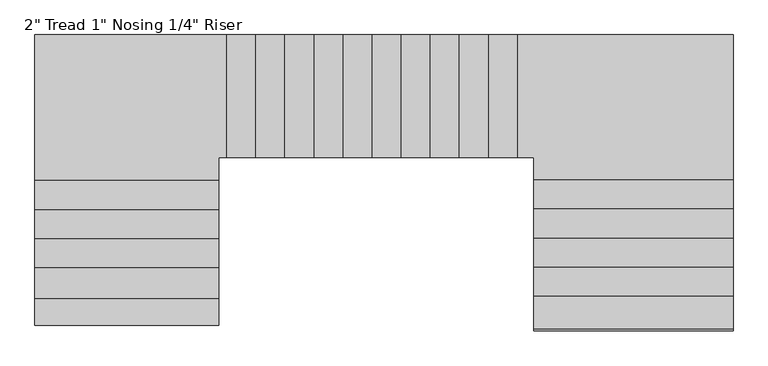
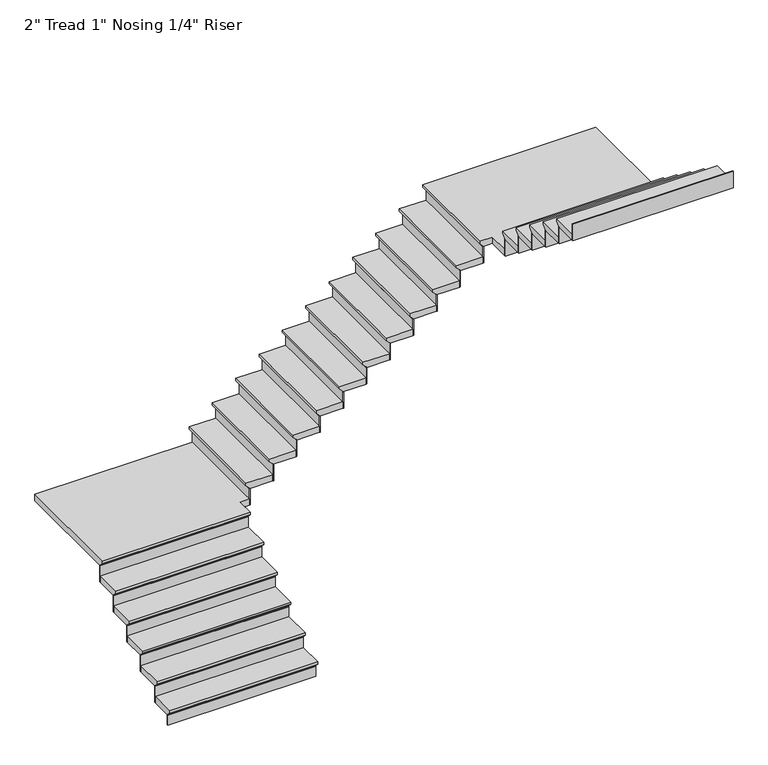
"""IFC4 building model written with IfcOpenShell, lengths in millimetres: stair flight geometry."""

from ifc_helpers import new_model, si_unit, origin, place, context, project, spatial, faceted_brep, source, transform, mapped, element, save


def stair_flight_6a7f422e(model_context):
    return source(origin(), model_context, "Body", "Brep", [
        faceted_brep([(-2368.6972892, 4718.9167606, 12915.0717391), (-2368.6972892, 4718.9167606, 12934.1217391), (-3493.0046642, 4718.9167606, 12934.1217391), (-3493.0046642, 4718.9167606, 12915.0717391), (-2368.6972892, 4744.3167606, 12889.6717391), (-3493.0046642, 4744.3167606, 12889.6717391), (-2368.6972892, 4909.4167606, 12934.1217391), (-3493.0046642, 4909.4167606, 12934.1217391), (-3493.0046642, 4744.3167606, 12883.3217391), (-3493.0046642, 4909.4167606, 12883.3217391), (-2368.6972892, 4909.4167606, 12883.3217391), (-2368.6972892, 4744.3167606, 12883.3217391)], [[[0, 1, 2, 3]], [[4, 0, 3, 5]], [[2, 1, 6, 7]], [[8, 9, 10, 11]], [[2, 7, 9, 8, 5, 3]], [[8, 11, 4, 5]], [[6, 1, 0, 4, 11, 10]], [[7, 6, 10, 9]]]),
        faceted_brep([(-2368.6972892, 4744.3167606, 12883.3217391), (-2368.6972892, 4744.3167606, 12801.6), (-2368.6972892, 4750.6667606, 12801.6), (-2368.6972892, 4750.6667606, 12883.3217391), (-3493.0046642, 4744.3167606, 12883.3217391), (-3493.0046642, 4750.6667606, 12883.3217391), (-3493.0046642, 4750.6667606, 12801.6), (-3493.0046642, 4744.3167606, 12801.6)], [[[0, 1, 2, 3]], [[4, 5, 6, 7]], [[1, 0, 4, 7]], [[2, 1, 7, 6]], [[3, 2, 6, 5]], [[0, 3, 5, 4]]]),
        faceted_brep([(-2368.6972892, 4909.4167606, 13015.8434783), (-2368.6972892, 4909.4167606, 12883.3217391), (-2368.6972892, 4915.7667606, 12883.3217391), (-2368.6972892, 4915.7667606, 13015.8434783), (-3493.0046642, 4909.4167606, 13015.8434783), (-3493.0046642, 4915.7667606, 13015.8434783), (-3493.0046642, 4915.7667606, 12883.3217391), (-3493.0046642, 4909.4167606, 12883.3217391)], [[[0, 1, 2, 3]], [[4, 5, 6, 7]], [[1, 0, 4, 7]], [[2, 1, 7, 6]], [[3, 2, 6, 5]], [[0, 3, 5, 4]]]),
        faceted_brep([(-3493.0046642, 4884.0167606, 13066.6434783), (-2368.6972892, 4884.0167606, 13066.6434783), (-2368.6972892, 5099.9164494, 13066.6434783), (-3493.0046642, 5099.9164494, 13066.6434783), (-3493.0046642, 4909.4167606, 13015.8434783), (-3493.0046642, 5099.9164494, 13015.8434783), (-2368.6972892, 5099.9164494, 13015.8434783), (-2368.6972892, 4909.4167606, 13015.8434783), (-3493.0046642, 4909.4167606, 13022.1934783), (-3493.0046642, 4884.0167606, 13047.5934783), (-2368.6972892, 4909.4167606, 13022.1934783), (-2368.6972892, 4884.0167606, 13047.5934783)], [[[0, 1, 2, 3]], [[4, 5, 6, 7]], [[0, 3, 5, 4, 8, 9]], [[4, 7, 10, 8]], [[2, 1, 11, 10, 7, 6]], [[3, 2, 6, 5]], [[11, 1, 0, 9]], [[10, 11, 9, 8]]]),
        faceted_brep([(-2368.6972892, 5099.9164494, 13148.3652174), (-2368.6972892, 5099.9164494, 13015.8434783), (-2368.6972892, 5106.2664494, 13015.8434783), (-2368.6972892, 5106.2664494, 13148.3652174), (-3493.0046642, 5099.9164494, 13148.3652174), (-3493.0046642, 5106.2664494, 13148.3652174), (-3493.0046642, 5106.2664494, 13015.8434783), (-3493.0046642, 5099.9164494, 13015.8434783)], [[[0, 1, 2, 3]], [[4, 5, 6, 7]], [[1, 0, 4, 7]], [[2, 1, 7, 6]], [[3, 2, 6, 5]], [[0, 3, 5, 4]]]),
        faceted_brep([(-3493.0046642, 5074.5164494, 13199.1652174), (-2368.6972892, 5074.5164494, 13199.1652174), (-2368.6972892, 5277.7164494, 13199.1652174), (-3493.0046642, 5277.7164494, 13199.1652174), (-3493.0046642, 5099.9164494, 13148.3652174), (-3493.0046642, 5277.7164494, 13148.3652174), (-2368.6972892, 5277.7164494, 13148.3652174), (-2368.6972892, 5099.9164494, 13148.3652174), (-3493.0046642, 5099.9164494, 13154.7152174), (-3493.0046642, 5074.5164494, 13180.1152174), (-2368.6972892, 5099.9164494, 13154.7152174), (-2368.6972892, 5074.5164494, 13180.1152174)], [[[0, 1, 2, 3]], [[4, 5, 6, 7]], [[0, 3, 5, 4, 8, 9]], [[4, 7, 10, 8]], [[2, 1, 11, 10, 7, 6]], [[3, 2, 6, 5]], [[11, 1, 0, 9]], [[10, 11, 9, 8]]]),
        faceted_brep([(-2368.6972892, 5277.7164494, 13280.8869565), (-2368.6972892, 5277.7164494, 13148.3652174), (-2368.6972892, 5284.0664494, 13148.3652174), (-2368.6972892, 5284.0664494, 13280.8869565), (-3493.0046642, 5277.7164494, 13280.8869565), (-3493.0046642, 5284.0664494, 13280.8869565), (-3493.0046642, 5284.0664494, 13148.3652174), (-3493.0046642, 5277.7164494, 13148.3652174)], [[[0, 1, 2, 3]], [[4, 5, 6, 7]], [[1, 0, 4, 7]], [[2, 1, 7, 6]], [[3, 2, 6, 5]], [[0, 3, 5, 4]]]),
        faceted_brep([(-3493.0046642, 5252.3164494, 13331.6869565), (-2368.6972892, 5252.3164494, 13331.6869565), (-2368.6972892, 5455.5164494, 13331.6869565), (-3493.0046642, 5455.5164494, 13331.6869565), (-3493.0046642, 5277.7164494, 13280.8869565), (-3493.0046642, 5455.5164494, 13280.8869565), (-2368.6972892, 5455.5164494, 13280.8869565), (-2368.6972892, 5277.7164494, 13280.8869565), (-3493.0046642, 5277.7164494, 13287.2369565), (-3493.0046642, 5252.3164494, 13312.6369565), (-2368.6972892, 5277.7164494, 13287.2369565), (-2368.6972892, 5252.3164494, 13312.6369565)], [[[0, 1, 2, 3]], [[4, 5, 6, 7]], [[0, 3, 5, 4, 8, 9]], [[4, 7, 10, 8]], [[2, 1, 11, 10, 7, 6]], [[3, 2, 6, 5]], [[11, 1, 0, 9]], [[10, 11, 9, 8]]]),
        faceted_brep([(-2368.6972892, 5455.5164494, 13413.4086957), (-2368.6972892, 5455.5164494, 13280.8869565), (-2368.6972892, 5461.8664494, 13280.8869565), (-2368.6972892, 5461.8664494, 13413.4086957), (-3493.0046642, 5455.5164494, 13413.4086957), (-3493.0046642, 5461.8664494, 13413.4086957), (-3493.0046642, 5461.8664494, 13280.8869565), (-3493.0046642, 5455.5164494, 13280.8869565)], [[[0, 1, 2, 3]], [[4, 5, 6, 7]], [[1, 0, 4, 7]], [[2, 1, 7, 6]], [[3, 2, 6, 5]], [[0, 3, 5, 4]]]),
        faceted_brep([(-3493.0046642, 5430.1164494, 13464.2086957), (-2368.6972892, 5430.1164494, 13464.2086957), (-2368.6972892, 5633.3167606, 13464.2086957), (-3493.0046642, 5633.3167606, 13464.2086957), (-3493.0046642, 5455.5164494, 13413.4086957), (-3493.0046642, 5633.3167606, 13413.4086957), (-2368.6972892, 5633.3167606, 13413.4086957), (-2368.6972892, 5455.5164494, 13413.4086957), (-3493.0046642, 5455.5164494, 13419.7586957), (-3493.0046642, 5430.1164494, 13445.1586957), (-2368.6972892, 5455.5164494, 13419.7586957), (-2368.6972892, 5430.1164494, 13445.1586957)], [[[0, 1, 2, 3]], [[4, 5, 6, 7]], [[0, 3, 5, 4, 8, 9]], [[4, 7, 10, 8]], [[2, 1, 11, 10, 7, 6]], [[3, 2, 6, 5]], [[11, 1, 0, 9]], [[10, 11, 9, 8]]]),
        faceted_brep([(-2368.6972892, 5633.3167606, 13545.9304348), (-2368.6972892, 5633.3167606, 13413.4086957), (-2368.6972892, 5639.6667606, 13413.4086957), (-2368.6972892, 5639.6667606, 13545.9304348), (-3493.0046642, 5633.3167606, 13545.9304348), (-3493.0046642, 5639.6667606, 13545.9304348), (-3493.0046642, 5639.6667606, 13413.4086957), (-3493.0046642, 5633.3167606, 13413.4086957)], [[[0, 1, 2, 3]], [[4, 5, 6, 7]], [[1, 0, 4, 7]], [[2, 1, 7, 6]], [[3, 2, 6, 5]], [[0, 3, 5, 4]]]),
        faceted_brep([(-2295.032382, 6496.9167606, 13596.7304348), (-3493.0046642, 6496.9167606, 13596.7304348), (-3493.0046642, 5607.9167606, 13596.7304348), (-2368.6972892, 5607.9167606, 13596.7304348), (-2368.6972892, 5746.5536537, 13596.7304348), (-2295.032382, 5746.5536537, 13596.7304348), (-3493.0046642, 6496.9167606, 13545.9304348), (-2295.032382, 6496.9167606, 13545.9304348), (-2295.032382, 5746.5536537, 13545.9304348), (-2368.6972892, 5746.5536537, 13545.9304348), (-2368.6972892, 5633.3167606, 13545.9304348), (-3493.0046642, 5633.3167606, 13545.9304348), (-3493.0046642, 5633.3167606, 13552.2804348), (-3493.0046642, 5607.9167606, 13577.6804348), (-2368.6972892, 5633.3167606, 13552.2804348), (-2368.6972892, 5607.9167606, 13577.6804348)], [[[0, 1, 2, 3, 4, 5]], [[6, 7, 8, 9, 10, 11]], [[1, 0, 7, 6]], [[2, 1, 6, 11, 12, 13]], [[11, 10, 14, 12]], [[4, 3, 15, 14, 10, 9]], [[5, 4, 9, 8]], [[0, 5, 8, 7]], [[15, 3, 2, 13]], [[14, 15, 13, 12]]]),
        faceted_brep([(-2295.032382, 5746.5536537, 13678.4521739), (-2295.032382, 5746.5536537, 13545.9304348), (-2288.682382, 5746.5536537, 13545.9304348), (-2288.682382, 5746.5536537, 13678.4521739), (-2295.032382, 6496.9167606, 13678.4521739), (-2288.682382, 6496.9167606, 13678.4521739), (-2288.682382, 6496.9167606, 13545.9304348), (-2295.032382, 6496.9167606, 13545.9304348)], [[[0, 1, 2, 3]], [[4, 5, 6, 7]], [[1, 0, 4, 7]], [[2, 1, 7, 6]], [[3, 2, 6, 5]], [[0, 3, 5, 4]]]),
        faceted_brep([(-2320.432382, 6496.9167606, 13729.2521739), (-2320.432382, 5746.5536537, 13729.2521739), (-2117.232382, 5746.5536537, 13729.2521739), (-2117.232382, 6496.9167606, 13729.2521739), (-2295.032382, 6496.9167606, 13678.4521739), (-2117.232382, 6496.9167606, 13678.4521739), (-2117.232382, 5746.5536537, 13678.4521739), (-2295.032382, 5746.5536537, 13678.4521739), (-2295.032382, 6496.9167606, 13684.8021739), (-2320.432382, 6496.9167606, 13710.2021739), (-2295.032382, 5746.5536537, 13684.8021739), (-2320.432382, 5746.5536537, 13710.2021739)], [[[0, 1, 2, 3]], [[4, 5, 6, 7]], [[0, 3, 5, 4, 8, 9]], [[4, 7, 10, 8]], [[2, 1, 11, 10, 7, 6]], [[3, 2, 6, 5]], [[11, 1, 0, 9]], [[10, 11, 9, 8]]]),
        faceted_brep([(-2117.232382, 5746.5536537, 13810.973913), (-2117.232382, 5746.5536537, 13678.4521739), (-2110.882382, 5746.5536537, 13678.4521739), (-2110.882382, 5746.5536537, 13810.973913), (-2117.232382, 6496.9167606, 13810.973913), (-2110.882382, 6496.9167606, 13810.973913), (-2110.882382, 6496.9167606, 13678.4521739), (-2117.232382, 6496.9167606, 13678.4521739)], [[[0, 1, 2, 3]], [[4, 5, 6, 7]], [[1, 0, 4, 7]], [[2, 1, 7, 6]], [[3, 2, 6, 5]], [[0, 3, 5, 4]]]),
        faceted_brep([(-2142.632382, 6496.9167606, 13861.773913), (-2142.632382, 5746.5536537, 13861.773913), (-1939.432382, 5746.5536537, 13861.773913), (-1939.432382, 6496.9167606, 13861.773913), (-2117.232382, 6496.9167606, 13810.973913), (-1939.432382, 6496.9167606, 13810.973913), (-1939.432382, 5746.5536537, 13810.973913), (-2117.232382, 5746.5536537, 13810.973913), (-2117.232382, 6496.9167606, 13817.323913), (-2142.632382, 6496.9167606, 13842.723913), (-2117.232382, 5746.5536537, 13817.323913), (-2142.632382, 5746.5536537, 13842.723913)], [[[0, 1, 2, 3]], [[4, 5, 6, 7]], [[0, 3, 5, 4, 8, 9]], [[4, 7, 10, 8]], [[2, 1, 11, 10, 7, 6]], [[3, 2, 6, 5]], [[11, 1, 0, 9]], [[10, 11, 9, 8]]]),
        faceted_brep([(-1939.432382, 5746.5536537, 13943.4956522), (-1939.432382, 5746.5536537, 13810.973913), (-1933.082382, 5746.5536537, 13810.973913), (-1933.082382, 5746.5536537, 13943.4956522), (-1939.432382, 6496.9167606, 13943.4956522), (-1933.082382, 6496.9167606, 13943.4956522), (-1933.082382, 6496.9167606, 13810.973913), (-1939.432382, 6496.9167606, 13810.973913)], [[[0, 1, 2, 3]], [[4, 5, 6, 7]], [[1, 0, 4, 7]], [[2, 1, 7, 6]], [[3, 2, 6, 5]], [[0, 3, 5, 4]]]),
        faceted_brep([(-1964.832382, 6496.9167606, 13994.2956522), (-1964.832382, 5746.5536537, 13994.2956522), (-1761.632382, 5746.5536537, 13994.2956522), (-1761.632382, 6496.9167606, 13994.2956522), (-1939.432382, 6496.9167606, 13943.4956522), (-1761.632382, 6496.9167606, 13943.4956522), (-1761.632382, 5746.5536537, 13943.4956522), (-1939.432382, 5746.5536537, 13943.4956522), (-1939.432382, 6496.9167606, 13949.8456522), (-1964.832382, 6496.9167606, 13975.2456522), (-1939.432382, 5746.5536537, 13949.8456522), (-1964.832382, 5746.5536537, 13975.2456522)], [[[0, 1, 2, 3]], [[4, 5, 6, 7]], [[0, 3, 5, 4, 8, 9]], [[4, 7, 10, 8]], [[2, 1, 11, 10, 7, 6]], [[3, 2, 6, 5]], [[11, 1, 0, 9]], [[10, 11, 9, 8]]]),
        faceted_brep([(-1761.632382, 5746.5536537, 14076.0173913), (-1761.632382, 5746.5536537, 13943.4956522), (-1755.282382, 5746.5536537, 13943.4956522), (-1755.282382, 5746.5536537, 14076.0173913), (-1761.632382, 6496.9167606, 14076.0173913), (-1755.282382, 6496.9167606, 14076.0173913), (-1755.282382, 6496.9167606, 13943.4956522), (-1761.632382, 6496.9167606, 13943.4956522)], [[[0, 1, 2, 3]], [[4, 5, 6, 7]], [[1, 0, 4, 7]], [[2, 1, 7, 6]], [[3, 2, 6, 5]], [[0, 3, 5, 4]]]),
        faceted_brep([(-1787.032382, 6496.9167606, 14126.8173913), (-1787.032382, 5746.5536537, 14126.8173913), (-1583.832382, 5746.5536537, 14126.8173913), (-1583.832382, 6496.9167606, 14126.8173913), (-1761.632382, 6496.9167606, 14076.0173913), (-1583.832382, 6496.9167606, 14076.0173913), (-1583.832382, 5746.5536537, 14076.0173913), (-1761.632382, 5746.5536537, 14076.0173913), (-1761.632382, 6496.9167606, 14082.3673913), (-1787.032382, 6496.9167606, 14107.7673913), (-1761.632382, 5746.5536537, 14082.3673913), (-1787.032382, 5746.5536537, 14107.7673913)], [[[0, 1, 2, 3]], [[4, 5, 6, 7]], [[0, 3, 5, 4, 8, 9]], [[4, 7, 10, 8]], [[2, 1, 11, 10, 7, 6]], [[3, 2, 6, 5]], [[11, 1, 0, 9]], [[10, 11, 9, 8]]]),
        faceted_brep([(-1583.832382, 5746.5536537, 14208.5391304), (-1583.832382, 5746.5536537, 14076.0173913), (-1577.482382, 5746.5536537, 14076.0173913), (-1577.482382, 5746.5536537, 14208.5391304), (-1583.832382, 6496.9167606, 14208.5391304), (-1577.482382, 6496.9167606, 14208.5391304), (-1577.482382, 6496.9167606, 14076.0173913), (-1583.832382, 6496.9167606, 14076.0173913)], [[[0, 1, 2, 3]], [[4, 5, 6, 7]], [[1, 0, 4, 7]], [[2, 1, 7, 6]], [[3, 2, 6, 5]], [[0, 3, 5, 4]]]),
        faceted_brep([(-1609.232382, 6496.9167606, 14259.3391304), (-1609.232382, 5746.5536537, 14259.3391304), (-1406.032382, 5746.5536537, 14259.3391304), (-1406.032382, 6496.9167606, 14259.3391304), (-1583.832382, 6496.9167606, 14208.5391304), (-1406.032382, 6496.9167606, 14208.5391304), (-1406.032382, 5746.5536537, 14208.5391304), (-1583.832382, 5746.5536537, 14208.5391304), (-1583.832382, 6496.9167606, 14214.8891304), (-1609.232382, 6496.9167606, 14240.2891304), (-1583.832382, 5746.5536537, 14214.8891304), (-1609.232382, 5746.5536537, 14240.2891304)], [[[0, 1, 2, 3]], [[4, 5, 6, 7]], [[0, 3, 5, 4, 8, 9]], [[4, 7, 10, 8]], [[2, 1, 11, 10, 7, 6]], [[3, 2, 6, 5]], [[11, 1, 0, 9]], [[10, 11, 9, 8]]]),
        faceted_brep([(-1406.032382, 5746.5536537, 14341.0608696), (-1406.032382, 5746.5536537, 14208.5391304), (-1399.682382, 5746.5536537, 14208.5391304), (-1399.682382, 5746.5536537, 14341.0608696), (-1406.032382, 6496.9167606, 14341.0608696), (-1399.682382, 6496.9167606, 14341.0608696), (-1399.682382, 6496.9167606, 14208.5391304), (-1406.032382, 6496.9167606, 14208.5391304)], [[[0, 1, 2, 3]], [[4, 5, 6, 7]], [[1, 0, 4, 7]], [[2, 1, 7, 6]], [[3, 2, 6, 5]], [[0, 3, 5, 4]]]),
        faceted_brep([(-1431.432382, 6496.9167606, 14391.8608696), (-1431.432382, 5746.5536537, 14391.8608696), (-1228.232382, 5746.5536537, 14391.8608696), (-1228.232382, 6496.9167606, 14391.8608696), (-1406.032382, 6496.9167606, 14341.0608696), (-1228.232382, 6496.9167606, 14341.0608696), (-1228.232382, 5746.5536537, 14341.0608696), (-1406.032382, 5746.5536537, 14341.0608696), (-1406.032382, 6496.9167606, 14347.4108696), (-1431.432382, 6496.9167606, 14372.8108696), (-1406.032382, 5746.5536537, 14347.4108696), (-1431.432382, 5746.5536537, 14372.8108696)], [[[0, 1, 2, 3]], [[4, 5, 6, 7]], [[0, 3, 5, 4, 8, 9]], [[4, 7, 10, 8]], [[2, 1, 11, 10, 7, 6]], [[3, 2, 6, 5]], [[11, 1, 0, 9]], [[10, 11, 9, 8]]]),
        faceted_brep([(-1228.232382, 5746.5536537, 14473.5826087), (-1228.232382, 5746.5536537, 14341.0608696), (-1221.882382, 5746.5536537, 14341.0608696), (-1221.882382, 5746.5536537, 14473.5826087), (-1228.232382, 6496.9167606, 14473.5826087), (-1221.882382, 6496.9167606, 14473.5826087), (-1221.882382, 6496.9167606, 14341.0608696), (-1228.232382, 6496.9167606, 14341.0608696)], [[[0, 1, 2, 3]], [[4, 5, 6, 7]], [[1, 0, 4, 7]], [[2, 1, 7, 6]], [[3, 2, 6, 5]], [[0, 3, 5, 4]]]),
        faceted_brep([(-1253.632382, 6496.9167606, 14524.3826087), (-1253.632382, 5746.5536537, 14524.3826087), (-1050.432382, 5746.5536537, 14524.3826087), (-1050.432382, 6496.9167606, 14524.3826087), (-1228.232382, 6496.9167606, 14473.5826087), (-1050.432382, 6496.9167606, 14473.5826087), (-1050.432382, 5746.5536537, 14473.5826087), (-1228.232382, 5746.5536537, 14473.5826087), (-1228.232382, 6496.9167606, 14479.9326087), (-1253.632382, 6496.9167606, 14505.3326087), (-1228.232382, 5746.5536537, 14479.9326087), (-1253.632382, 5746.5536537, 14505.3326087)], [[[0, 1, 2, 3]], [[4, 5, 6, 7]], [[0, 3, 5, 4, 8, 9]], [[4, 7, 10, 8]], [[2, 1, 11, 10, 7, 6]], [[3, 2, 6, 5]], [[11, 1, 0, 9]], [[10, 11, 9, 8]]]),
        faceted_brep([(-1050.432382, 5746.5536537, 14606.1043478), (-1050.432382, 5746.5536537, 14473.5826087), (-1044.082382, 5746.5536537, 14473.5826087), (-1044.082382, 5746.5536537, 14606.1043478), (-1050.432382, 6496.9167606, 14606.1043478), (-1044.082382, 6496.9167606, 14606.1043478), (-1044.082382, 6496.9167606, 14473.5826087), (-1050.432382, 6496.9167606, 14473.5826087)], [[[0, 1, 2, 3]], [[4, 5, 6, 7]], [[1, 0, 4, 7]], [[2, 1, 7, 6]], [[3, 2, 6, 5]], [[0, 3, 5, 4]]]),
        faceted_brep([(-1075.832382, 6496.9167606, 14656.9043478), (-1075.832382, 5746.5536537, 14656.9043478), (-872.632382, 5746.5536537, 14656.9043478), (-872.632382, 6496.9167606, 14656.9043478), (-1050.432382, 6496.9167606, 14606.1043478), (-872.632382, 6496.9167606, 14606.1043478), (-872.632382, 5746.5536537, 14606.1043478), (-1050.432382, 5746.5536537, 14606.1043478), (-1050.432382, 6496.9167606, 14612.4543478), (-1075.832382, 6496.9167606, 14637.8543478), (-1050.432382, 5746.5536537, 14612.4543478), (-1075.832382, 5746.5536537, 14637.8543478)], [[[0, 1, 2, 3]], [[4, 5, 6, 7]], [[0, 3, 5, 4, 8, 9]], [[4, 7, 10, 8]], [[2, 1, 11, 10, 7, 6]], [[3, 2, 6, 5]], [[11, 1, 0, 9]], [[10, 11, 9, 8]]]),
        faceted_brep([(-872.632382, 5746.5536537, 14738.626087), (-872.632382, 5746.5536537, 14606.1043478), (-866.282382, 5746.5536537, 14606.1043478), (-866.282382, 5746.5536537, 14738.626087), (-872.632382, 6496.9167606, 14738.626087), (-866.282382, 6496.9167606, 14738.626087), (-866.282382, 6496.9167606, 14606.1043478), (-872.632382, 6496.9167606, 14606.1043478)], [[[0, 1, 2, 3]], [[4, 5, 6, 7]], [[1, 0, 4, 7]], [[2, 1, 7, 6]], [[3, 2, 6, 5]], [[0, 3, 5, 4]]]),
        faceted_brep([(-898.032382, 6496.9167606, 14789.426087), (-898.032382, 5746.5536537, 14789.426087), (-694.832382, 5746.5536537, 14789.426087), (-694.832382, 6496.9167606, 14789.426087), (-872.632382, 6496.9167606, 14738.626087), (-694.832382, 6496.9167606, 14738.626087), (-694.832382, 5746.5536537, 14738.626087), (-872.632382, 5746.5536537, 14738.626087), (-872.632382, 6496.9167606, 14744.976087), (-898.032382, 6496.9167606, 14770.376087), (-872.632382, 5746.5536537, 14744.976087), (-898.032382, 5746.5536537, 14770.376087)], [[[0, 1, 2, 3]], [[4, 5, 6, 7]], [[0, 3, 5, 4, 8, 9]], [[4, 7, 10, 8]], [[2, 1, 11, 10, 7, 6]], [[3, 2, 6, 5]], [[11, 1, 0, 9]], [[10, 11, 9, 8]]]),
        faceted_brep([(-694.832382, 5746.5536537, 14871.1478261), (-694.832382, 5746.5536537, 14738.626087), (-688.482382, 5746.5536537, 14738.626087), (-688.482382, 5746.5536537, 14871.1478261), (-694.832382, 6496.9167606, 14871.1478261), (-688.482382, 6496.9167606, 14871.1478261), (-688.482382, 6496.9167606, 14738.626087), (-694.832382, 6496.9167606, 14738.626087)], [[[0, 1, 2, 3]], [[4, 5, 6, 7]], [[1, 0, 4, 7]], [[2, 1, 7, 6]], [[3, 2, 6, 5]], [[0, 3, 5, 4]]]),
        faceted_brep([(-720.232382, 6496.9167606, 14921.9478261), (-720.232382, 5746.5536537, 14921.9478261), (-517.032382, 5746.5536537, 14921.9478261), (-517.032382, 6496.9167606, 14921.9478261), (-694.832382, 6496.9167606, 14871.1478261), (-517.032382, 6496.9167606, 14871.1478261), (-517.032382, 5746.5536537, 14871.1478261), (-694.832382, 5746.5536537, 14871.1478261), (-694.832382, 6496.9167606, 14877.4978261), (-720.232382, 6496.9167606, 14902.8978261), (-694.832382, 5746.5536537, 14877.4978261), (-720.232382, 5746.5536537, 14902.8978261)], [[[0, 1, 2, 3]], [[4, 5, 6, 7]], [[0, 3, 5, 4, 8, 9]], [[4, 7, 10, 8]], [[2, 1, 11, 10, 7, 6]], [[3, 2, 6, 5]], [[11, 1, 0, 9]], [[10, 11, 9, 8]]]),
        faceted_brep([(-517.032382, 5746.5536537, 15003.6695652), (-517.032382, 5746.5536537, 14871.1478261), (-510.682382, 5746.5536537, 14871.1478261), (-510.682382, 5746.5536537, 15003.6695652), (-517.032382, 6496.9167606, 15003.6695652), (-510.682382, 6496.9167606, 15003.6695652), (-510.682382, 6496.9167606, 14871.1478261), (-517.032382, 6496.9167606, 14871.1478261)], [[[0, 1, 2, 3]], [[4, 5, 6, 7]], [[1, 0, 4, 7]], [[2, 1, 7, 6]], [[3, 2, 6, 5]], [[0, 3, 5, 4]]]),
        faceted_brep([(774.1953358, 5582.5167606, 15054.4695652), (774.1953358, 6496.9167606, 15054.4695652), (-542.432382, 6496.9167606, 15054.4695652), (-542.432382, 5746.5536537, 15054.4695652), (-445.0046642, 5746.5536537, 15054.4695652), (-445.0046642, 5582.5167606, 15054.4695652), (774.1953358, 6496.9167606, 15003.6695652), (774.1953358, 5582.5167606, 15003.6695652), (-445.0046642, 5582.5167606, 15003.6695652), (-445.0046642, 5746.5536537, 15003.6695652), (-517.032382, 5746.5536537, 15003.6695652), (-517.032382, 6496.9167606, 15003.6695652), (-517.032382, 6496.9167606, 15010.0195652), (-542.432382, 6496.9167606, 15035.4195652), (-517.032382, 5746.5536537, 15010.0195652), (-542.432382, 5746.5536537, 15035.4195652)], [[[0, 1, 2, 3, 4, 5]], [[6, 7, 8, 9, 10, 11]], [[1, 0, 7, 6]], [[2, 1, 6, 11, 12, 13]], [[11, 10, 14, 12]], [[4, 3, 15, 14, 10, 9]], [[5, 4, 9, 8]], [[0, 5, 8, 7]], [[15, 3, 2, 13]], [[14, 15, 13, 12]]]),
        faceted_brep([(-445.0046642, 5582.5167606, 15136.1913043), (-445.0046642, 5582.5167606, 15003.6695652), (-445.0046642, 5576.1667606, 15003.6695652), (-445.0046642, 5576.1667606, 15136.1913043), (774.1953358, 5582.5167606, 15136.1913043), (774.1953358, 5576.1667606, 15136.1913043), (774.1953358, 5576.1667606, 15003.6695652), (774.1953358, 5582.5167606, 15003.6695652)], [[[0, 1, 2, 3]], [[4, 5, 6, 7]], [[1, 0, 4, 7]], [[2, 1, 7, 6]], [[3, 2, 6, 5]], [[0, 3, 5, 4]]]),
        faceted_brep([(774.1953358, 5607.9167606, 15186.9913043), (-445.0046642, 5607.9167606, 15186.9913043), (-445.0046642, 5404.7164494, 15186.9913043), (774.1953358, 5404.7164494, 15186.9913043), (774.1953358, 5582.5167606, 15136.1913043), (774.1953358, 5404.7164494, 15136.1913043), (-445.0046642, 5404.7164494, 15136.1913043), (-445.0046642, 5582.5167606, 15136.1913043), (774.1953358, 5582.5167606, 15142.5413043), (774.1953358, 5607.9167606, 15167.9413043), (-445.0046642, 5582.5167606, 15142.5413043), (-445.0046642, 5607.9167606, 15167.9413043)], [[[0, 1, 2, 3]], [[4, 5, 6, 7]], [[0, 3, 5, 4, 8, 9]], [[4, 7, 10, 8]], [[2, 1, 11, 10, 7, 6]], [[3, 2, 6, 5]], [[11, 1, 0, 9]], [[10, 11, 9, 8]]]),
        faceted_brep([(-445.0046642, 5404.7164494, 15268.7130435), (-445.0046642, 5404.7164494, 15136.1913043), (-445.0046642, 5398.3664494, 15136.1913043), (-445.0046642, 5398.3664494, 15268.7130435), (774.1953358, 5404.7164494, 15268.7130435), (774.1953358, 5398.3664494, 15268.7130435), (774.1953358, 5398.3664494, 15136.1913043), (774.1953358, 5404.7164494, 15136.1913043)], [[[0, 1, 2, 3]], [[4, 5, 6, 7]], [[1, 0, 4, 7]], [[2, 1, 7, 6]], [[3, 2, 6, 5]], [[0, 3, 5, 4]]]),
        faceted_brep([(774.1953358, 5430.1164494, 15319.5130435), (-445.0046642, 5430.1164494, 15319.5130435), (-445.0046642, 5226.9164494, 15319.5130435), (774.1953358, 5226.9164494, 15319.5130435), (774.1953358, 5404.7164494, 15268.7130435), (774.1953358, 5226.9164494, 15268.7130435), (-445.0046642, 5226.9164494, 15268.7130435), (-445.0046642, 5404.7164494, 15268.7130435), (774.1953358, 5404.7164494, 15275.0630435), (774.1953358, 5430.1164494, 15300.4630435), (-445.0046642, 5404.7164494, 15275.0630435), (-445.0046642, 5430.1164494, 15300.4630435)], [[[0, 1, 2, 3]], [[4, 5, 6, 7]], [[0, 3, 5, 4, 8, 9]], [[4, 7, 10, 8]], [[2, 1, 11, 10, 7, 6]], [[3, 2, 6, 5]], [[11, 1, 0, 9]], [[10, 11, 9, 8]]]),
        faceted_brep([(-445.0046642, 5226.9164494, 15401.2347826), (-445.0046642, 5226.9164494, 15268.7130435), (-445.0046642, 5220.5664494, 15268.7130435), (-445.0046642, 5220.5664494, 15401.2347826), (774.1953358, 5226.9164494, 15401.2347826), (774.1953358, 5220.5664494, 15401.2347826), (774.1953358, 5220.5664494, 15268.7130435), (774.1953358, 5226.9164494, 15268.7130435)], [[[0, 1, 2, 3]], [[4, 5, 6, 7]], [[1, 0, 4, 7]], [[2, 1, 7, 6]], [[3, 2, 6, 5]], [[0, 3, 5, 4]]]),
        faceted_brep([(774.1953358, 5252.3164494, 15452.0347826), (-445.0046642, 5252.3164494, 15452.0347826), (-445.0046642, 5049.1164494, 15452.0347826), (774.1953358, 5049.1164494, 15452.0347826), (774.1953358, 5226.9164494, 15401.2347826), (774.1953358, 5049.1164494, 15401.2347826), (-445.0046642, 5049.1164494, 15401.2347826), (-445.0046642, 5226.9164494, 15401.2347826), (774.1953358, 5226.9164494, 15407.5847826), (774.1953358, 5252.3164494, 15432.9847826), (-445.0046642, 5226.9164494, 15407.5847826), (-445.0046642, 5252.3164494, 15432.9847826)], [[[0, 1, 2, 3]], [[4, 5, 6, 7]], [[0, 3, 5, 4, 8, 9]], [[4, 7, 10, 8]], [[2, 1, 11, 10, 7, 6]], [[3, 2, 6, 5]], [[11, 1, 0, 9]], [[10, 11, 9, 8]]]),
        faceted_brep([(-445.0046642, 5049.1164494, 15533.7565217), (-445.0046642, 5049.1164494, 15401.2347826), (-445.0046642, 5042.7664494, 15401.2347826), (-445.0046642, 5042.7664494, 15533.7565217), (774.1953358, 5049.1164494, 15533.7565217), (774.1953358, 5042.7664494, 15533.7565217), (774.1953358, 5042.7664494, 15401.2347826), (774.1953358, 5049.1164494, 15401.2347826)], [[[0, 1, 2, 3]], [[4, 5, 6, 7]], [[1, 0, 4, 7]], [[2, 1, 7, 6]], [[3, 2, 6, 5]], [[0, 3, 5, 4]]]),
        faceted_brep([(774.1953358, 5074.5164494, 15584.5565217), (-445.0046642, 5074.5164494, 15584.5565217), (-445.0046642, 4871.3164494, 15584.5565217), (774.1953358, 4871.3164494, 15584.5565217), (774.1953358, 5049.1164494, 15533.7565217), (774.1953358, 4871.3164494, 15533.7565217), (-445.0046642, 4871.3164494, 15533.7565217), (-445.0046642, 5049.1164494, 15533.7565217), (774.1953358, 5049.1164494, 15540.1065217), (774.1953358, 5074.5164494, 15565.5065217), (-445.0046642, 5049.1164494, 15540.1065217), (-445.0046642, 5074.5164494, 15565.5065217)], [[[0, 1, 2, 3]], [[4, 5, 6, 7]], [[0, 3, 5, 4, 8, 9]], [[4, 7, 10, 8]], [[2, 1, 11, 10, 7, 6]], [[3, 2, 6, 5]], [[11, 1, 0, 9]], [[10, 11, 9, 8]]]),
        faceted_brep([(-445.0046642, 4871.3164494, 15666.2782609), (-445.0046642, 4871.3164494, 15533.7565217), (-445.0046642, 4864.9664494, 15533.7565217), (-445.0046642, 4864.9664494, 15666.2782609), (774.1953358, 4871.3164494, 15666.2782609), (774.1953358, 4864.9664494, 15666.2782609), (774.1953358, 4864.9664494, 15533.7565217), (774.1953358, 4871.3164494, 15533.7565217)], [[[0, 1, 2, 3]], [[4, 5, 6, 7]], [[1, 0, 4, 7]], [[2, 1, 7, 6]], [[3, 2, 6, 5]], [[0, 3, 5, 4]]]),
        faceted_brep([(-445.0046642, 4693.5167606, 15798.8), (-445.0046642, 4693.5167606, 15666.2782609), (-445.0046642, 4687.1667606, 15666.2782609), (-445.0046642, 4687.1667606, 15798.8), (774.1953358, 4693.5167606, 15798.8), (774.1953358, 4687.1667606, 15798.8), (774.1953358, 4687.1667606, 15666.2782609), (774.1953358, 4693.5167606, 15666.2782609)], [[[0, 1, 2, 3]], [[4, 5, 6, 7]], [[1, 0, 4, 7]], [[2, 1, 7, 6]], [[3, 2, 6, 5]], [[0, 3, 5, 4]]]),
        faceted_brep([(774.1953358, 4896.7164494, 15717.0782609), (-445.0046642, 4896.7164494, 15717.0782609), (-445.0046642, 4693.5167606, 15717.0782609), (774.1953358, 4693.5167606, 15717.0782609), (774.1953358, 4871.3164494, 15666.2782609), (774.1953358, 4693.5167606, 15666.2782609), (-445.0046642, 4693.5167606, 15666.2782609), (-445.0046642, 4871.3164494, 15666.2782609), (774.1953358, 4871.3164494, 15672.6282609), (774.1953358, 4896.7164494, 15698.0282609), (-445.0046642, 4871.3164494, 15672.6282609), (-445.0046642, 4896.7164494, 15698.0282609)], [[[0, 1, 2, 3]], [[4, 5, 6, 7]], [[0, 3, 5, 4, 8, 9]], [[4, 7, 10, 8]], [[2, 1, 11, 10, 7, 6]], [[3, 2, 6, 5]], [[11, 1, 0, 9]], [[10, 11, 9, 8]]]),
    ])


if __name__ == "__main__":
    model = new_model("IFC4")
    model_context = context("Model", 3, world=origin())
    ifc_project = project(units=[si_unit("LENGTHUNIT", "METRE", prefix="MILLI")], contexts=[model_context])
    site = spatial("IfcSite", under=ifc_project)
    building = spatial("IfcBuilding", under=site)
    placement = place(None, origin())
    stair_flight_shape = stair_flight_6a7f422e(model_context)
    element("IfcStairFlight", 1, ObjectType="2\" Tread 1\" Nosing 1/4\" Riser", at=placement, inside=building, context=model_context, shape_type="MappedRepresentation", body=[
        mapped(stair_flight_shape, transform((0.0, 0.0, 0.0), x_axis=(1.0, 0.0, 0.0), y_axis=(0.0, 1.0, 0.0), z_axis=(0.0, 0.0, 1.0))),
    ])
    save(model, "model.ifc")
